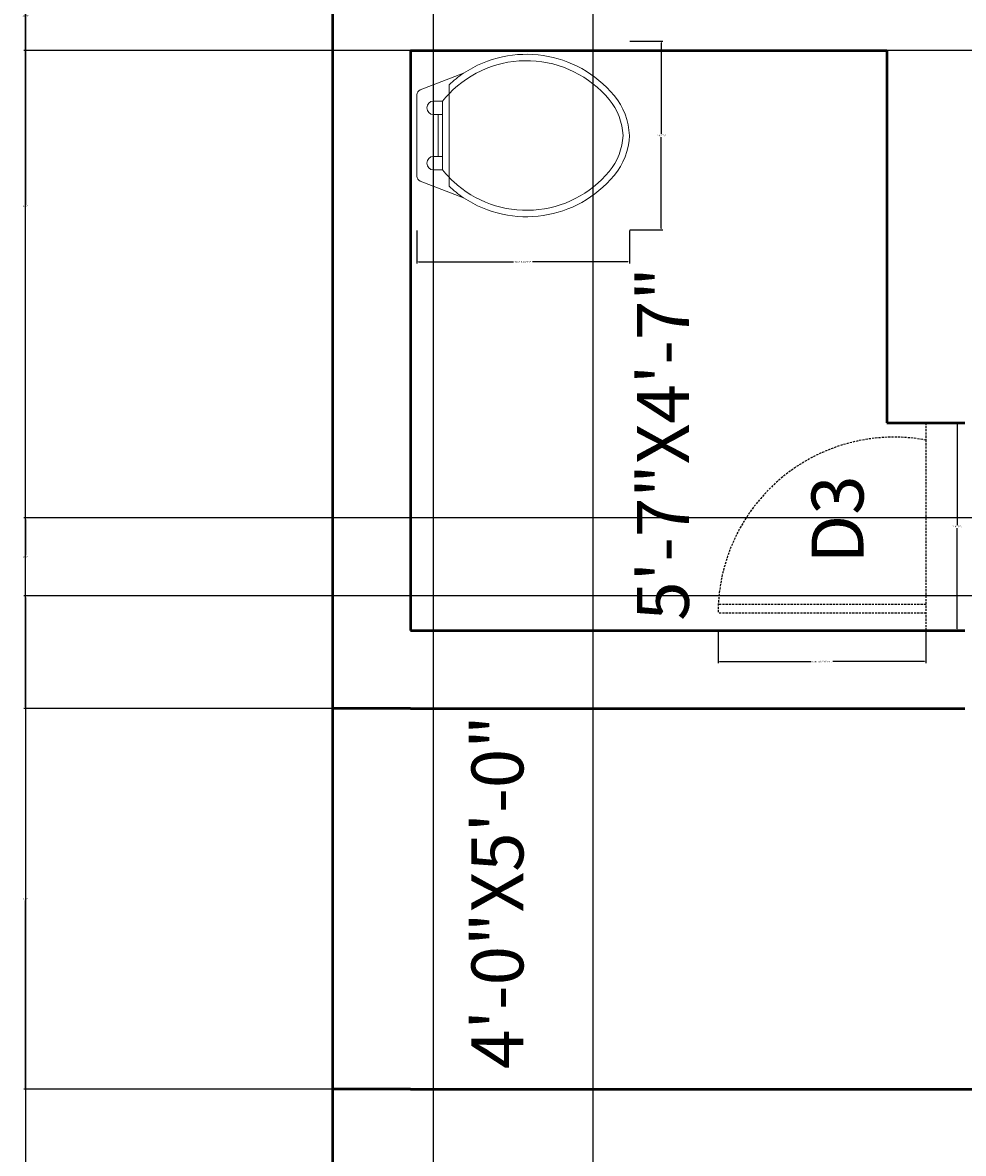
# Model space of a CAD drawing. Units: inches. Extents: x 3 to 576, y -689 to 51.
# Tile 4 of 21: x 3 to 111, y -514 to -383. Entities that reach past the tile are written whole.
import ezdxf

# ---------------------------------------------------------------- set-up
doc = ezdxf.new("R2010")
doc.units = ezdxf.units.IN
doc.header["$MEASUREMENT"] = 0
doc.linetypes.add('DASHED2', pattern=[0.375, 0.25, -0.125])
for name, color, linetype, lineweight in [('A-ANNO-DIMS', 2, 'Continuous', 18), ('A-ANNO-TEXT', 3, 'Continuous', 18), ('A-AREA-IDEN', 7, 'Continuous', 18), ('A-DOOR', 4, 'DASHED2', 25), ('A-FLOR-FIXT', 9, 'Continuous', 18), ('A-WALL', 7, 'Continuous', 50)]:
    doc.layers.add(name, color=color, linetype=linetype, lineweight=lineweight)
doc.styles.get("Standard").update_dxf_attribs({"font": 'arial.ttf'})
doc.dimstyles.get("Standard").update_dxf_attribs({"dimtxt": 0.18, "dimasz": 0.18, "dimexe": 0.18, "dimexo": 0.0625, "dimgap": 0.09, "dimtad": 0, "dimtih": 1, "dimtoh": 1, "dimdec": 0, "dimzin": 0, "dimdsep": 46, "dimlunit": 3, "dimtxsty": 'Standard', "dimcen": 0.09, "dimadec": 0, "dimazin": 0, "dimtfac": 1, "dimtdec": 0, "dimtofl": 0, "dimtmove": 0, "dimatfit": 3, "dimfxl": 1, "dimtolj": 1, "dimtzin": 0, "dimarcsym": 0})

# ---------------------------------------------------------------- blocks, each defined once
blk = doc.blocks.new('WC')
for p, q in [((3.72, 14.21), (3.72, 15.24)), ((3.72, 14.21), (3.72, 9.38)), ((3.72, 4.55), (3.72, 9.38)), ((3.72, 3.52), (3.72, 4.55))]:
    blk.add_line(p, q)
for points in [[(5.4, 16.57, -0.383919), (22.78, 13.99, -0.163732), (24.55, 9.38, -0.359733)], [(3.72, 14.21, -0.448546), (22.21, 13.53, -0.162618), (23.81, 9.38, -0.470877)], [(0, 9.38), (0, 14.07, -0.31031), (0.39, 14.64), (5.4, 16.57, -0.209071)], [(3.72, 15.24, -0.040937), (5.4, 16.57, -0.163732)], [(2.98, 13.36), (1.94, 13.36, 1), (1.94, 11.8), (2.48, 11.8)], [(2.98, 13.36, -0.022712), (3.72, 14.21, -0.162618)], [(2.98, 9.38), (2.98, 13.36, -0.476108)], [(0, 9.38), (0, 4.69, 0.31031), (0.39, 4.12), (5.4, 2.19, 0.209071)], [(2.98, 9.38), (2.98, 5.4, 0.022712)], [(4.22, 4.06, 0.431639), (22.21, 5.23, 0.162618), (23.81, 9.38, 0.470877)], [(5.4, 2.19, 0.383919), (22.78, 4.76, 0.163732), (24.55, 9.38, 0.359733)], [(2.98, 5.4), (1.94, 5.4, -1), (1.94, 6.96), (2.48, 6.96)], [(2.98, 5.4, 0.022712), (3.72, 4.55, 0.162618)], [(3.72, 4.55, 0.014165), (4.22, 4.06, 0.162618)], [(3.72, 3.52, 0.040937), (5.4, 2.19, 0.163732)]]:
    blk.add_lwpolyline(points, format="xyb")
for points in [[(2.48, 11.8), (2.48, 6.96)], [(2.48, 11.8), (2.98, 11.8)], [(2.48, 6.96), (2.98, 6.96)]]:
    blk.add_lwpolyline(points)
blk = doc.blocks.new('DOOR-750')
for p, q in [((24, 24), (24, 22)), ((24, 22), (24, 0)), ((24, 2), (0, 2))]:
    blk.add_line(p, q)
blk.add_arc((20.33, 2), 20.33, 79.6111, 180)
blk = doc.blocks.new('*D19')
at = {"layer": 'A-ANNO-DIMS', "color": 0, "lineweight": -2, "transparency": 16777216}
for p, q in [((48.01, -407.11), (48.01, -410.91)), ((72.56, -407.11), (72.56, -410.91)), ((48.19, -410.73), (59.19, -410.73)), ((72.38, -410.73), (61.38, -410.73))]:
    blk.add_line(p, q, dxfattribs=at)
at = {"layer": 'A-ANNO-DIMS', "color": 0, "transparency": 16777216}
for points in [[(48.19, -410.7), (48.19, -410.76), (48.01, -410.73)], [(72.38, -410.7), (72.38, -410.76), (72.56, -410.73)]]:
    blk.add_solid(points, dxfattribs=at)
at = {"layer": 'Defpoints', "color": 0, "transparency": 16777216}
for p in [(48.01, -407.05), (72.56, -407.05), (72.56, -410.73)]:
    blk.add_point(p, dxfattribs=at)
at = {"layer": 'A-ANNO-DIMS', "color": 0, "transparency": 16777216, "insert": (60.29, -410.73), "char_height": 0.18, "attachment_point": 5}
blk.add_mtext('\\A1;WC 2\'-0 1/2" TYP.', dxfattribs=at)
blk = doc.blocks.new('*D20')
at = {"layer": 'A-ANNO-DIMS', "color": 0, "lineweight": -2, "transparency": 16777216}
for p, q in [((72.62, -385.24), (76.42, -385.24)), ((76.24, -385.42), (76.24, -395.96)), ((76.24, -406.87), (76.24, -396.33)), ((72.62, -407.05), (76.42, -407.05))]:
    blk.add_line(p, q, dxfattribs=at)
at = {"layer": 'A-ANNO-DIMS', "color": 0, "transparency": 16777216}
for points in [[(76.21, -385.42), (76.27, -385.42), (76.24, -385.24)], [(76.21, -406.87), (76.27, -406.87), (76.24, -407.05)]]:
    blk.add_solid(points, dxfattribs=at)
at = {"layer": 'Defpoints', "color": 0, "transparency": 16777216}
for p in [(72.56, -385.24), (76.24, -385.24), (72.56, -407.05)]:
    blk.add_point(p, dxfattribs=at)
at = {"layer": 'A-ANNO-DIMS', "color": 0, "transparency": 16777216, "insert": (76.24, -396.15), "char_height": 0.18, "attachment_point": 5}
blk.add_mtext('\\A1;1\'-10" TYP.', dxfattribs=at)
blk = doc.blocks.new('*D29')
at = {"layer": 'A-ANNO-DIMS', "color": 0, "lineweight": -2, "transparency": 16777216}
for p, q in [((82.79, -453.37), (82.79, -457.09)), ((106.79, -453.37), (106.79, -457.09)), ((82.97, -456.91), (93.55, -456.91)), ((106.61, -456.91), (96.04, -456.91))]:
    blk.add_line(p, q, dxfattribs=at)
at = {"layer": 'A-ANNO-DIMS', "color": 0, "transparency": 16777216}
for points in [[(82.97, -456.88), (82.97, -456.94), (82.79, -456.91)], [(106.61, -456.88), (106.61, -456.94), (106.79, -456.91)]]:
    blk.add_solid(points, dxfattribs=at)
at = {"layer": 'Defpoints', "color": 0, "transparency": 16777216}
for p in [(82.79, -453.31), (106.79, -453.31), (106.79, -456.91)]:
    blk.add_point(p, dxfattribs=at)
at = {"layer": 'A-ANNO-DIMS', "color": 0, "transparency": 16777216, "insert": (94.79, -456.91), "char_height": 0.18, "attachment_point": 5}
blk.add_mtext('\\A1;DOOR D3 2\'-0" TYP.', dxfattribs=at)
blk = doc.blocks.new('*D30')
at = {"layer": 'A-ANNO-DIMS', "color": 0, "lineweight": -2, "transparency": 16777216}
for p, q in [((106.86, -429.31), (110.57, -429.31)), ((110.39, -429.49), (110.39, -441.13)), ((110.39, -453.13), (110.39, -441.49)), ((106.86, -453.31), (110.57, -453.31))]:
    blk.add_line(p, q, dxfattribs=at)
at = {"layer": 'A-ANNO-DIMS', "color": 0, "transparency": 16777216}
for points in [[(110.36, -429.49), (110.42, -429.49), (110.39, -429.31)], [(110.36, -453.13), (110.42, -453.13), (110.39, -453.31)]]:
    blk.add_solid(points, dxfattribs=at)
at = {"layer": 'Defpoints', "color": 0, "transparency": 16777216}
for p in [(106.79, -429.31), (110.39, -429.31), (106.79, -453.31)]:
    blk.add_point(p, dxfattribs=at)
at = {"layer": 'A-ANNO-DIMS', "color": 0, "transparency": 16777216, "insert": (110.39, -441.31), "char_height": 0.18, "attachment_point": 5}
blk.add_mtext('\\A1;2\'-0" TYP.', dxfattribs=at)
blk = doc.blocks.new('*D58')
at = {"layer": 'A-ANNO-DIMS', "color": 0, "lineweight": -2, "transparency": 16777216}
for p, q in [((47.23, -302.31), (2.66, -302.31)), ((2.84, -302.49), (2.84, -382.13)), ((2.84, -462.13), (2.84, -382.49)), ((38.23, -462.31), (2.66, -462.31))]:
    blk.add_line(p, q, dxfattribs=at)
at = {"layer": 'A-ANNO-DIMS', "color": 0, "transparency": 16777216}
for points in [[(2.81, -302.49), (2.87, -302.49), (2.84, -302.31)], [(2.81, -462.13), (2.87, -462.13), (2.84, -462.31)]]:
    blk.add_solid(points, dxfattribs=at)
at = {"layer": 'Defpoints', "color": 0, "transparency": 16777216}
for p in [(47.29, -302.31), (2.84, -462.31), (38.29, -462.31)]:
    blk.add_point(p, dxfattribs=at)
at = {"layer": 'A-ANNO-DIMS', "color": 0, "transparency": 16777216, "insert": (2.84, -382.31), "char_height": 0.18, "attachment_point": 5}
blk.add_mtext('\\A1;13\'-4"', dxfattribs=at)
blk = doc.blocks.new('*D59')
at = {"layer": 'A-ANNO-DIMS', "color": 0, "lineweight": -2, "transparency": 16777216}
for p, q in [((38.23, -462.31), (2.66, -462.31)), ((2.84, -462.49), (2.84, -484.13)), ((2.84, -506.13), (2.84, -484.49)), ((38.23, -506.31), (2.66, -506.31))]:
    blk.add_line(p, q, dxfattribs=at)
at = {"layer": 'A-ANNO-DIMS', "color": 0, "transparency": 16777216}
for points in [[(2.81, -462.49), (2.87, -462.49), (2.84, -462.31)], [(2.81, -506.13), (2.87, -506.13), (2.84, -506.31)]]:
    blk.add_solid(points, dxfattribs=at)
at = {"layer": 'Defpoints', "color": 0, "transparency": 16777216}
for p in [(38.29, -462.31), (2.84, -506.31), (38.29, -506.31)]:
    blk.add_point(p, dxfattribs=at)
at = {"layer": 'A-ANNO-DIMS', "color": 0, "transparency": 16777216, "insert": (2.84, -484.31), "char_height": 0.18, "attachment_point": 5}
blk.add_mtext('\\A1;3\'-8"', dxfattribs=at)
blk = doc.blocks.new('*D60')
at = {"layer": 'A-ANNO-DIMS', "color": 0, "lineweight": -2, "transparency": 16777216}
for p, q in [((38.23, -506.31), (2.66, -506.31)), ((2.84, -506.49), (2.84, -551.13)), ((2.84, -596.13), (2.84, -551.49)), ((47.23, -596.31), (2.66, -596.31))]:
    blk.add_line(p, q, dxfattribs=at)
at = {"layer": 'A-ANNO-DIMS', "color": 0, "transparency": 16777216}
for points in [[(2.81, -506.49), (2.87, -506.49), (2.84, -506.31)], [(2.81, -596.13), (2.87, -596.13), (2.84, -596.31)]]:
    blk.add_solid(points, dxfattribs=at)
at = {"layer": 'Defpoints', "color": 0, "transparency": 16777216}
for p in [(38.29, -506.31), (2.84, -596.31), (47.29, -596.31)]:
    blk.add_point(p, dxfattribs=at)
at = {"layer": 'A-ANNO-DIMS', "color": 0, "transparency": 16777216, "insert": (2.84, -551.31), "char_height": 0.18, "attachment_point": 5}
blk.add_mtext('\\A1;7\'-6"', dxfattribs=at)
blk = doc.blocks.new('*D71')
at = {"layer": 'A-ANNO-DIMS', "color": 0, "lineweight": -2, "transparency": 16777216}
for p, q in [((531.23, -368.31), (2.66, -368.31)), ((2.84, -368.49), (2.84, -404.13)), ((2.84, -440.13), (2.84, -404.49)), ((531.23, -440.31), (2.66, -440.31))]:
    blk.add_line(p, q, dxfattribs=at)
at = {"layer": 'A-ANNO-DIMS', "color": 0, "transparency": 16777216}
for points in [[(2.81, -368.49), (2.87, -368.49), (2.84, -368.31)], [(2.81, -440.13), (2.87, -440.13), (2.84, -440.31)]]:
    blk.add_solid(points, dxfattribs=at)
at = {"layer": 'Defpoints', "color": 0, "transparency": 16777216}
for p in [(531.29, -368.31), (2.84, -440.31), (531.29, -440.31)]:
    blk.add_point(p, dxfattribs=at)
at = {"layer": 'A-ANNO-DIMS', "color": 0, "transparency": 16777216, "insert": (2.84, -404.31), "char_height": 0.18, "attachment_point": 5}
blk.add_mtext('\\A1;6\'-0"', dxfattribs=at)
blk = doc.blocks.new('*D72')
at = {"layer": 'A-ANNO-DIMS', "color": 0, "lineweight": -2, "transparency": 16777216}
for p, q in [((531.23, -440.31), (2.66, -440.31)), ((2.84, -440.49), (2.84, -444.63)), ((2.84, -449.13), (2.84, -444.99)), ((531.23, -449.31), (2.66, -449.31))]:
    blk.add_line(p, q, dxfattribs=at)
at = {"layer": 'A-ANNO-DIMS', "color": 0, "transparency": 16777216}
for points in [[(2.81, -440.49), (2.87, -440.49), (2.84, -440.31)], [(2.81, -449.13), (2.87, -449.13), (2.84, -449.31)]]:
    blk.add_solid(points, dxfattribs=at)
at = {"layer": 'Defpoints', "color": 0, "transparency": 16777216}
for p in [(531.29, -440.31), (2.84, -449.31), (531.29, -449.31)]:
    blk.add_point(p, dxfattribs=at)
at = {"layer": 'A-ANNO-DIMS', "color": 0, "transparency": 16777216, "insert": (2.84, -444.81), "char_height": 0.18, "attachment_point": 5}
blk.add_mtext('\\A1;0\'-9"', dxfattribs=at)
blk = doc.blocks.new('*D73')
at = {"layer": 'A-ANNO-DIMS', "color": 0, "lineweight": -2, "transparency": 16777216}
for p, q in [((531.23, -449.31), (2.66, -449.31)), ((2.84, -449.49), (2.84, -518.13)), ((2.84, -587.13), (2.84, -518.49)), ((531.23, -587.31), (2.66, -587.31))]:
    blk.add_line(p, q, dxfattribs=at)
at = {"layer": 'A-ANNO-DIMS', "color": 0, "transparency": 16777216}
for points in [[(2.81, -449.49), (2.87, -449.49), (2.84, -449.31)], [(2.81, -587.13), (2.87, -587.13), (2.84, -587.31)]]:
    blk.add_solid(points, dxfattribs=at)
at = {"layer": 'Defpoints', "color": 0, "transparency": 16777216}
for p in [(531.29, -449.31), (2.84, -587.31), (531.29, -587.31)]:
    blk.add_point(p, dxfattribs=at)
at = {"layer": 'A-ANNO-DIMS', "color": 0, "transparency": 16777216, "insert": (2.84, -518.31), "char_height": 0.18, "attachment_point": 5}
blk.add_mtext('\\A1;11\'-6"', dxfattribs=at)
blk = doc.blocks.new('*D121')
at = {"layer": 'A-ANNO-DIMS', "color": 0, "lineweight": -2, "transparency": 16777216}
for p, q in [((49.91, -350.9), (49.91, -688.94)), ((68.33, -356.2), (68.33, -688.94)), ((50.09, -688.76), (58.59, -688.76)), ((68.15, -688.76), (59.65, -688.76))]:
    blk.add_line(p, q, dxfattribs=at)
at = {"layer": 'A-ANNO-DIMS', "color": 0, "transparency": 16777216}
for points in [[(50.09, -688.73), (50.09, -688.79), (49.91, -688.76)], [(68.15, -688.73), (68.15, -688.79), (68.33, -688.76)]]:
    blk.add_solid(points, dxfattribs=at)
at = {"layer": 'Defpoints', "color": 0, "transparency": 16777216}
for p in [(49.91, -350.84), (68.33, -356.14), (68.33, -688.76)]:
    blk.add_point(p, dxfattribs=at)
at = {"layer": 'A-ANNO-DIMS', "color": 0, "transparency": 16777216, "insert": (59.12, -688.76), "char_height": 0.18, "attachment_point": 5}
blk.add_mtext('\\A1;1\'-6 1/2"', dxfattribs=at)
blk = doc.blocks.new('*D125')
at = {"layer": 'A-ANNO-DIMS', "color": 0, "lineweight": -2, "transparency": 16777216}
for p, q in [((531.23, -368.31), (2.66, -368.31)), ((2.84, -368.49), (2.84, -377.13)), ((2.84, -386.13), (2.84, -377.49)), ((512.45, -386.31), (2.66, -386.31))]:
    blk.add_line(p, q, dxfattribs=at)
at = {"layer": 'A-ANNO-DIMS', "color": 0, "transparency": 16777216}
for points in [[(2.81, -368.49), (2.87, -368.49), (2.84, -368.31)], [(2.81, -386.13), (2.87, -386.13), (2.84, -386.31)]]:
    blk.add_solid(points, dxfattribs=at)
at = {"layer": 'Defpoints', "color": 0, "transparency": 16777216}
for p in [(531.29, -368.31), (2.84, -386.31), (512.51, -386.31)]:
    blk.add_point(p, dxfattribs=at)
at = {"layer": 'A-ANNO-DIMS', "color": 0, "transparency": 16777216, "insert": (2.84, -377.31), "char_height": 0.18, "attachment_point": 5}
blk.add_mtext('\\A1;1\'-6"', dxfattribs=at)

msp = doc.modelspace()

# ---------------------------------------------------------------- linework, layer by layer
at = {"layer": 'A-DOOR'}
msp.add_line((106.79, -450.31), (82.79, -450.31), dxfattribs=at)
at = {"layer": 'A-WALL'}
for p, q in [((38.29, 15.69), (38.29, -653.31)), ((47.29, -386.31), (102.29, -386.31)), ((47.29, -386.31), (47.29, -453.31)), ((102.29, -386.31), (102.29, -429.31)), ((102.29, -429.31), (111.29, -429.31)), ((47.29, -453.31), (111.29, -453.31)), ((47.29, -462.31), (38.29, -462.31)), ((47.29, -462.31), (111.29, -462.31)), ((47.29, -506.31), (38.29, -506.31)), ((47.29, -506.31), (255.29, -506.31))]:
    msp.add_line(p, q, dxfattribs=at)

# ---------------------------------------------------------------- block references
at = {"layer": 'A-DOOR'}
msp.add_blockref('DOOR-750', (82.79, -453.31), dxfattribs=at)
at = {"layer": 'A-FLOR-FIXT'}
msp.add_blockref('WC', (48.01, -405.52), dxfattribs=at)

# ---------------------------------------------------------------- texts
at = {"layer": 'A-ANNO-TEXT', "insert": (93.58, -445.58), "char_height": 6, "attachment_point": 1, "rotation": 90}
msp.add_mtext('D3', dxfattribs=at)
at = {"layer": 'A-AREA-IDEN', "insert": (73.42, -452.19), "char_height": 6, "attachment_point": 1, "rotation": 90}
msp.add_mtext_dynamic_manual_height_columns('5\'-7"X4\'-7"', width=0.9477, gutter_width=1, heights=[0], dxfattribs=at)
at = {"layer": 'A-AREA-IDEN', "insert": (54.32, -503.96), "char_height": 6, "attachment_point": 1, "rotation": 90}
msp.add_mtext('4\'-0"X5\'-0"', dxfattribs=at)

# ---------------------------------------------------------------- dimensions: what is measured, and where the dimension line sits
at = {"layer": 'A-ANNO-DIMS'}
for base, p1, p2, picture, middle in [((2.84, -462.31), (47.29, -302.31), (38.29, -462.31), '*D58', (2.84, -382.31)), ((2.84, -440.31), (531.29, -368.31), (531.29, -440.31), '*D71', (2.84, -404.31)), ((2.84, -386.31), (531.29, -368.31), (512.51, -386.31), '*D125', (2.84, -377.31)), ((2.84, -449.31), (531.29, -440.31), (531.29, -449.31), '*D72', (2.84, -444.81)), ((2.84, -587.31), (531.29, -449.31), (531.29, -587.31), '*D73', (2.84, -518.31)), ((2.84, -506.31), (38.29, -462.31), (38.29, -506.31), '*D59', (2.84, -484.31)), ((2.84, -596.31), (38.29, -506.31), (47.29, -596.31), '*D60', (2.84, -551.31))]:
    dim = msp.add_linear_dim(base=base, p1=p1, p2=p2, angle=90, dimstyle='Standard', override={"dimdec": 1, "dimlfac": 1, "dimrnd": 0, "dimzin": 1, "dimdsep": 46, "dimlunit": 4, "dimfrac": 2}, dxfattribs=at)
    dim.commit()
    dim.dimension.update_dxf_attribs({"geometry": picture, "text_midpoint": middle})
dim = msp.add_linear_dim(base=(68.33, -688.76), p1=(49.91, -350.84), p2=(68.33, -356.14), dimstyle='Standard', override={"dimdec": 1, "dimlfac": 1, "dimrnd": 0, "dimzin": 1, "dimdsep": 46, "dimlunit": 4, "dimfrac": 2}, dxfattribs=at)
dim.commit()
dim.dimension.update_dxf_attribs({"geometry": '*D121', "text_midpoint": (59.12, -688.76)})
for base, p1, p2, picture, middle in [((76.24, -385.24), (72.56, -407.05), (72.56, -385.24), '*D20', (76.24, -396.15)), ((110.39, -429.31), (106.79, -453.31), (106.79, -429.31), '*D30', (110.39, -441.31))]:
    dim = msp.add_linear_dim(base=base, p1=p1, p2=p2, angle=90, text='<> TYP.', dimstyle='Standard', override={"dimdec": 1, "dimlfac": 1, "dimrnd": 0, "dimzin": 1, "dimdsep": 46, "dimlunit": 4, "dimfrac": 2}, dxfattribs=at)
    dim.commit()
    dim.dimension.update_dxf_attribs({"geometry": picture, "text_midpoint": middle})
for base, p1, p2, text, picture, middle in [((72.5614, -410.7322), (48.0137, -407.05), (72.5614, -407.05), 'WC <> TYP.', '*D19', (60.2875, -410.7322)), ((106.79, -456.91), (82.79, -453.31), (106.79, -453.31), 'DOOR D3 <> TYP.', '*D29', (94.79, -456.91))]:
    dim = msp.add_linear_dim(base=base, p1=p1, p2=p2, text=text, dimstyle='Standard', override={"dimdec": 1, "dimlfac": 1, "dimrnd": 0, "dimzin": 1, "dimdsep": 46, "dimlunit": 4, "dimfrac": 2}, dxfattribs=at)
    dim.commit()
    dim.dimension.update_dxf_attribs({"geometry": picture, "text_midpoint": middle})

doc.saveas('drawing.dxf')
